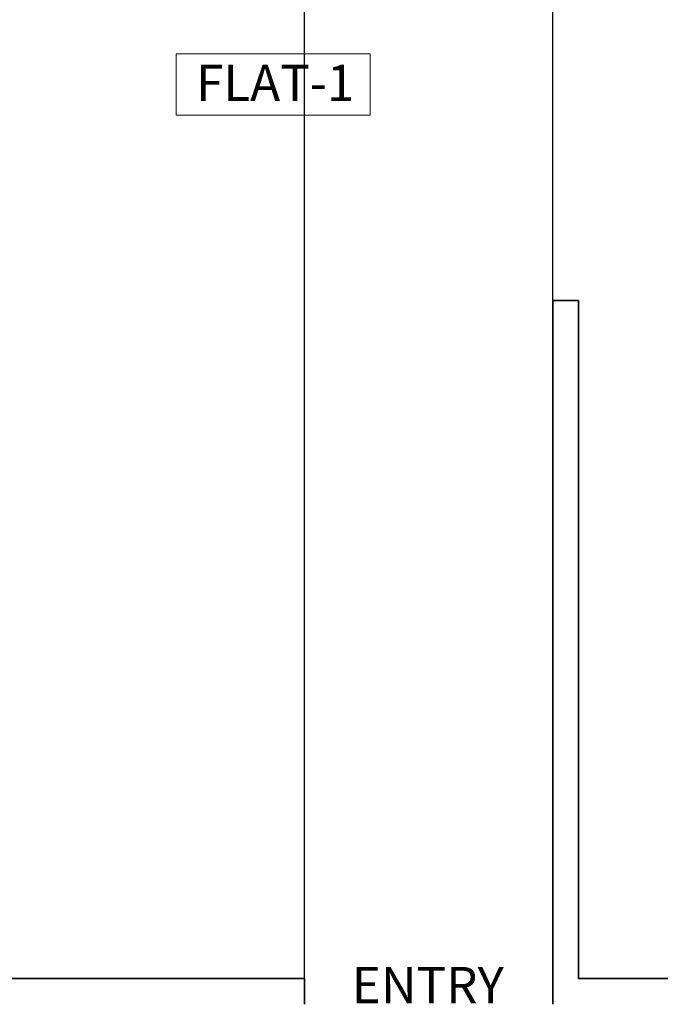
# Model space of a CAD drawing. Units: inches. Extents: x 3731 to 4318, y 1310 to 2388.
# Tile 41 of 57: x 4000 to 4124, y 1938 to 2129. Entities that reach past the tile are written whole.
import ezdxf

# ---------------------------------------------------------------- set-up
doc = ezdxf.new("R2010")
doc.units = ezdxf.units.IN
for name, color, linetype, lineweight in [('A-ANNO-DIMS', 2, 'Continuous', 18), ('A-ANNO-TEXT', 7, 'Continuous', 18), ('A-AREA-IDEN', 7, 'Continuous', 18), ('A-WALL', 7, 'Continuous', 35)]:
    doc.layers.add(name, color=color, linetype=linetype, lineweight=lineweight)
doc.styles.get("Standard").update_dxf_attribs({"font": 'arial.ttf'})
doc.dimstyles.get("Standard").update_dxf_attribs({"dimtxt": 0.18, "dimasz": 0.18, "dimexe": 0.18, "dimexo": 0.0625, "dimgap": 0.09, "dimtad": 0, "dimtih": 1, "dimtoh": 1, "dimdec": 4, "dimzin": 0, "dimdsep": 46, "dimtxsty": 'Standard', "dimcen": 0.09, "dimadec": 0, "dimazin": 0, "dimtfac": 1, "dimtdec": 4, "dimtofl": 0, "dimtmove": 0, "dimatfit": 3, "dimfxl": 1, "dimtolj": 1, "dimtzin": 0, "dimarcsym": 0})

# ---------------------------------------------------------------- blocks, each defined once
blk = doc.blocks.new('*D38')
at = {"layer": 'A-ANNO-DIMS', "color": 0, "lineweight": -2, "transparency": 16777216}
for p, q in [((4103.27, 2262.38), (4318.34, 2262.38)), ((4318.16, 2262.2), (4318.16, 2103.06)), ((4318.16, 1943.56), (4318.16, 2102.7)), ((4234.27, 1943.38), (4318.34, 1943.38))]:
    blk.add_line(p, q, dxfattribs=at)
at = {"layer": 'A-ANNO-DIMS', "color": 0, "transparency": 16777216}
for points in [[(4318.13, 2262.2), (4318.19, 2262.2), (4318.16, 2262.38)], [(4318.13, 1943.56), (4318.19, 1943.56), (4318.16, 1943.38)]]:
    blk.add_solid(points, dxfattribs=at)
at = {"layer": 'Defpoints', "color": 0, "transparency": 16777216}
for p in [(4103.21, 2262.38), (4318.16, 2262.38), (4234.21, 1943.38)]:
    blk.add_point(p, dxfattribs=at)
at = {"layer": 'A-ANNO-DIMS', "color": 0, "transparency": 16777216, "insert": (4318.16, 2102.88), "char_height": 0.18, "attachment_point": 5}
blk.add_mtext('\\A1;319', dxfattribs=at)
blk = doc.blocks.new('*D49')
at = {"layer": 'A-ANNO-DIMS', "color": 0, "lineweight": -2, "transparency": 16777216}
for p, q in [((4055.21, 1943.44), (4055.21, 2387.51)), ((4055.39, 2387.33), (4078.99, 2387.33)), ((4103.03, 2387.33), (4079.43, 2387.33)), ((4103.21, 1938.44), (4103.21, 2387.51))]:
    blk.add_line(p, q, dxfattribs=at)
at = {"layer": 'A-ANNO-DIMS', "color": 0, "transparency": 16777216}
for points in [[(4055.39, 2387.36), (4055.39, 2387.3), (4055.21, 2387.33)], [(4103.03, 2387.36), (4103.03, 2387.3), (4103.21, 2387.33)]]:
    blk.add_solid(points, dxfattribs=at)
at = {"layer": 'Defpoints', "color": 0, "transparency": 16777216}
for p in [(4103.21, 2387.33), (4055.21, 1943.38), (4103.21, 1938.38)]:
    blk.add_point(p, dxfattribs=at)
at = {"layer": 'A-ANNO-DIMS', "color": 0, "transparency": 16777216, "insert": (4079.21, 2387.33), "char_height": 0.18, "attachment_point": 5}
blk.add_mtext('\\A1;48', dxfattribs=at)

msp = doc.modelspace()

# ---------------------------------------------------------------- linework, layer by layer
at = {"layer": 'A-AREA-IDEN'}
msp.add_lwpolyline([(4030.41, 2122.08), (4067.95, 2122.08), (4067.95, 2110.17), (4030.41, 2110.17)], close=True, dxfattribs=at)
at = {"layer": 'A-WALL'}
for p, q in [((4103.21, 2074.38), (4103.21, 1938.38)), ((4103.21, 2074.38), (4108.21, 2074.38)), ((4108.21, 2074.38), (4108.21, 1943.38)), ((3840.21, 1943.38), (4055.21, 1943.38)), ((4055.21, 1938.38), (4055.21, 1943.38)), ((4108.21, 1943.38), (4234.21, 1943.38))]:
    msp.add_line(p, q, dxfattribs=at)

# ---------------------------------------------------------------- texts
at = {"layer": 'A-ANNO-TEXT', "insert": (4064.37, 1945.6), "char_height": 7, "attachment_point": 1}
msp.add_mtext_dynamic_manual_height_columns('ENTRY', width=10.4564, gutter_width=12.5, heights=[0], dxfattribs=at)
at = {"layer": 'A-AREA-IDEN', "insert": (4034.26, 2119.94), "char_height": 7, "attachment_point": 1}
msp.add_mtext_dynamic_manual_height_columns('FLAT-1', width=24.0878, gutter_width=12.5, heights=[0], dxfattribs=at)

# ---------------------------------------------------------------- dimensions: what is measured, and where the dimension line sits
at = {"layer": 'A-ANNO-DIMS'}
dim = msp.add_linear_dim(base=(4103.21, 2387.33), p1=(4055.21, 1943.38), p2=(4103.21, 1938.38), dimstyle='Standard', override={"dimdec": 0, "dimlfac": 1, "dimrnd": 0, "dimzin": 0, "dimdsep": 46, "dimlunit": 2}, dxfattribs=at)
dim.commit()
dim.dimension.update_dxf_attribs({"geometry": '*D49', "text_midpoint": (4079.21, 2387.33)})
dim = msp.add_linear_dim(base=(4318.16, 2262.38), p1=(4234.21, 1943.38), p2=(4103.21, 2262.38), angle=90, dimstyle='Standard', override={"dimdec": 0, "dimlfac": 1, "dimrnd": 0, "dimzin": 0, "dimdsep": 46, "dimlunit": 2}, dxfattribs=at)
dim.commit()
dim.dimension.update_dxf_attribs({"geometry": '*D38', "text_midpoint": (4318.16, 2102.88)})

doc.saveas('drawing.dxf')
